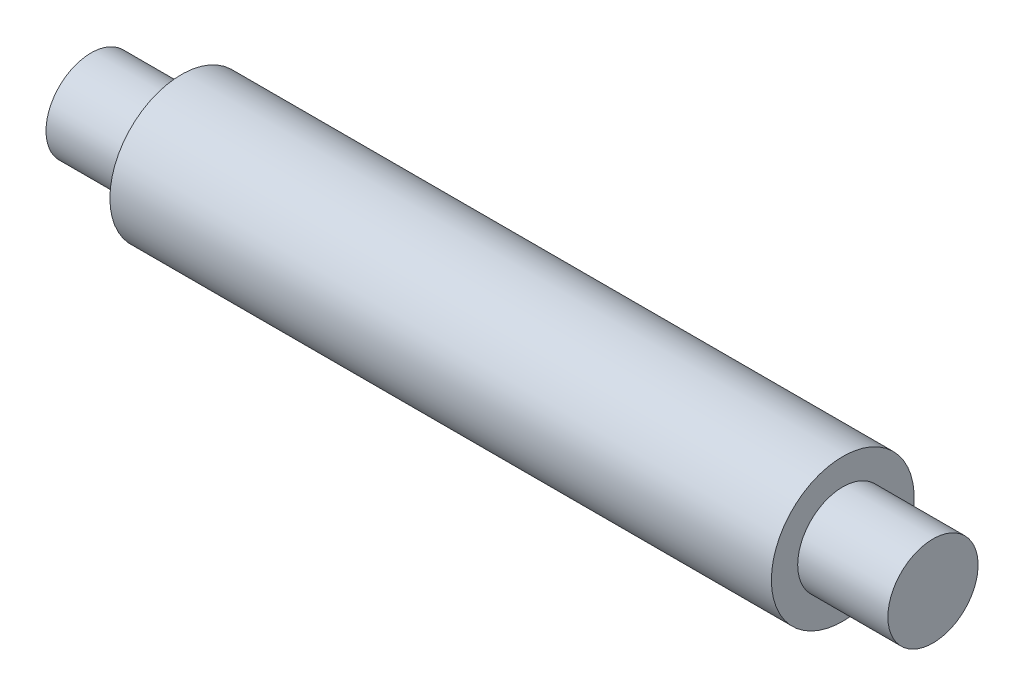
ISO-10303-21;
HEADER;
FILE_DESCRIPTION(('STEP AP214'),'2;1');
FILE_NAME('part.step','',(''),(''),'','','');
FILE_SCHEMA(('AUTOMOTIVE_DESIGN { 1 0 10303 214 1 1 1 1 }'));
ENDSEC;
DATA;
#1=APPLICATION_CONTEXT('core data for automotive mechanical design processes');
#2=APPLICATION_PROTOCOL_DEFINITION('international standard','automotive_design',2000,#1);
#3=PRODUCT_CONTEXT('',#1,'mechanical');
#4=PRODUCT('Part','Part','',(#3));
#5=PRODUCT_RELATED_PRODUCT_CATEGORY('part','',(#4));
#6=PRODUCT_DEFINITION_FORMATION('','',#4);
#7=PRODUCT_DEFINITION_CONTEXT('part definition',#1,'design');
#8=PRODUCT_DEFINITION('design','',#6,#7);
#9=PRODUCT_DEFINITION_SHAPE('','',#8);
#10=(LENGTH_UNIT() NAMED_UNIT(*) SI_UNIT(.MILLI.,.METRE.));
#11=(NAMED_UNIT(*) PLANE_ANGLE_UNIT() SI_UNIT($,.RADIAN.));
#12=(NAMED_UNIT(*) SI_UNIT($,.STERADIAN.) SOLID_ANGLE_UNIT());
#13=UNCERTAINTY_MEASURE_WITH_UNIT(LENGTH_MEASURE(1.E-05),#10,'distance_accuracy_value','');
#14=(GEOMETRIC_REPRESENTATION_CONTEXT(3) GLOBAL_UNCERTAINTY_ASSIGNED_CONTEXT((#13)) GLOBAL_UNIT_ASSIGNED_CONTEXT((#10,
#11,#12)) REPRESENTATION_CONTEXT('',''));
#15=CARTESIAN_POINT('',(0.,0.,0.));
#16=DIRECTION('',(0.,0.,1.));
#17=DIRECTION('',(1.,0.,0.));
#18=AXIS2_PLACEMENT_3D('',#15,#16,#17);
#19=CARTESIAN_POINT('',(280.,30.0000000000002,0.));
#20=DIRECTION('',(1.,0.,0.));
#21=DIRECTION('',(0.,0.,-1.));
#22=AXIS2_PLACEMENT_3D('',#19,#20,#21);
#23=PLANE('',#22);
#24=CARTESIAN_POINT('',(280.,0.,0.));
#25=DIRECTION('',(-1.,0.,0.));
#26=DIRECTION('',(0.,0.,1.));
#27=AXIS2_PLACEMENT_3D('',#24,#25,#26);
#28=CIRCLE('',#27,30.0000000000002);
#29=CARTESIAN_POINT('',(280.,0.,30.0000000000002));
#30=VERTEX_POINT('',#29);
#31=EDGE_CURVE('E10',#30,#30,#28,.T.);
#32=ORIENTED_EDGE('',*,*,#31,.F.);
#33=EDGE_LOOP('',(#32));
#34=FACE_BOUND('',#33,.T.);
#35=ADVANCED_FACE('F36',(#34),#23,.T.);
#36=CARTESIAN_POINT('',(-409.616293782747,0.,0.));
#37=DIRECTION('',(-1.,0.,0.));
#38=DIRECTION('',(0.,0.,1.));
#39=AXIS2_PLACEMENT_3D('',#36,#37,#38);
#40=CYLINDRICAL_SURFACE('',#39,30.0000000000002);
#41=ORIENTED_EDGE('',*,*,#31,.T.);
#42=EDGE_LOOP('',(#41));
#43=FACE_BOUND('',#42,.T.);
#44=CARTESIAN_POINT('',(220.,0.,0.));
#45=DIRECTION('',(-1.,0.,0.));
#46=DIRECTION('',(0.,0.,1.));
#47=AXIS2_PLACEMENT_3D('',#44,#45,#46);
#48=CIRCLE('',#47,30.0000000000002);
#49=CARTESIAN_POINT('',(220.,0.,30.0000000000002));
#50=VERTEX_POINT('',#49);
#51=EDGE_CURVE('E46',#50,#50,#48,.T.);
#52=ORIENTED_EDGE('',*,*,#51,.F.);
#53=EDGE_LOOP('',(#52));
#54=FACE_BOUND('',#53,.T.);
#55=ADVANCED_FACE('F142',(#43,#54),#40,.T.);
#56=CARTESIAN_POINT('',(220.,47.5000000000001,0.));
#57=DIRECTION('',(1.,0.,0.));
#58=DIRECTION('',(0.,0.,-1.));
#59=AXIS2_PLACEMENT_3D('',#56,#57,#58);
#60=PLANE('',#59);
#61=ORIENTED_EDGE('',*,*,#51,.T.);
#62=EDGE_LOOP('',(#61));
#63=FACE_BOUND('',#62,.T.);
#64=CARTESIAN_POINT('',(220.,0.,0.));
#65=DIRECTION('',(-1.,0.,0.));
#66=DIRECTION('',(0.,0.,1.));
#67=AXIS2_PLACEMENT_3D('',#64,#65,#66);
#68=CIRCLE('',#67,47.5000000000001);
#69=CARTESIAN_POINT('',(220.,0.,47.5000000000001));
#70=VERTEX_POINT('',#69);
#71=EDGE_CURVE('E49',#70,#70,#68,.T.);
#72=ORIENTED_EDGE('',*,*,#71,.F.);
#73=EDGE_LOOP('',(#72));
#74=FACE_BOUND('',#73,.T.);
#75=ADVANCED_FACE('F138',(#63,#74),#60,.T.);
#76=CARTESIAN_POINT('',(-409.616293782747,0.,0.));
#77=DIRECTION('',(-1.,0.,0.));
#78=DIRECTION('',(0.,0.,1.));
#79=AXIS2_PLACEMENT_3D('',#76,#77,#78);
#80=CYLINDRICAL_SURFACE('',#79,47.5);
#81=ORIENTED_EDGE('',*,*,#71,.T.);
#82=EDGE_LOOP('',(#81));
#83=FACE_BOUND('',#82,.T.);
#84=CARTESIAN_POINT('',(-220.,0.,0.));
#85=DIRECTION('',(-1.,0.,0.));
#86=DIRECTION('',(0.,0.,1.));
#87=AXIS2_PLACEMENT_3D('',#84,#85,#86);
#88=CIRCLE('',#87,47.4999999999999);
#89=CARTESIAN_POINT('',(-220.,0.,47.4999999999999));
#90=VERTEX_POINT('',#89);
#91=EDGE_CURVE('E53',#90,#90,#88,.T.);
#92=ORIENTED_EDGE('',*,*,#91,.F.);
#93=EDGE_LOOP('',(#92));
#94=FACE_BOUND('',#93,.T.);
#95=ADVANCED_FACE('F133',(#83,#94),#80,.T.);
#96=CARTESIAN_POINT('',(-220.,47.4999999999999,0.));
#97=DIRECTION('',(-1.,0.,0.));
#98=DIRECTION('',(0.,0.,1.));
#99=AXIS2_PLACEMENT_3D('',#96,#97,#98);
#100=PLANE('',#99);
#101=ORIENTED_EDGE('',*,*,#91,.T.);
#102=EDGE_LOOP('',(#101));
#103=FACE_BOUND('',#102,.T.);
#104=CARTESIAN_POINT('',(-220.,0.,0.));
#105=DIRECTION('',(-1.,0.,0.));
#106=DIRECTION('',(0.,0.,1.));
#107=AXIS2_PLACEMENT_3D('',#104,#105,#106);
#108=CIRCLE('',#107,29.9999999999999);
#109=CARTESIAN_POINT('',(-220.,0.,29.9999999999999));
#110=VERTEX_POINT('',#109);
#111=EDGE_CURVE('E56',#110,#110,#108,.T.);
#112=ORIENTED_EDGE('',*,*,#111,.F.);
#113=EDGE_LOOP('',(#112));
#114=FACE_BOUND('',#113,.T.);
#115=ADVANCED_FACE('F128',(#103,#114),#100,.T.);
#116=CARTESIAN_POINT('',(-409.616293782747,0.,0.));
#117=DIRECTION('',(-1.,0.,0.));
#118=DIRECTION('',(0.,0.,1.));
#119=AXIS2_PLACEMENT_3D('',#116,#117,#118);
#120=CYLINDRICAL_SURFACE('',#119,29.9999999999999);
#121=ORIENTED_EDGE('',*,*,#111,.T.);
#122=EDGE_LOOP('',(#121));
#123=FACE_BOUND('',#122,.T.);
#124=CARTESIAN_POINT('',(-280.,0.,0.));
#125=DIRECTION('',(-1.,0.,0.));
#126=DIRECTION('',(0.,0.,1.));
#127=AXIS2_PLACEMENT_3D('',#124,#125,#126);
#128=CIRCLE('',#127,29.9999999999999);
#129=CARTESIAN_POINT('',(-280.,0.,29.9999999999999));
#130=VERTEX_POINT('',#129);
#131=EDGE_CURVE('E65',#130,#130,#128,.T.);
#132=ORIENTED_EDGE('',*,*,#131,.F.);
#133=EDGE_LOOP('',(#132));
#134=FACE_BOUND('',#133,.T.);
#135=ADVANCED_FACE('F127',(#123,#134),#120,.T.);
#136=CARTESIAN_POINT('',(-280.,29.9999999999999,0.));
#137=DIRECTION('',(-1.,0.,0.));
#138=DIRECTION('',(0.,0.,1.));
#139=AXIS2_PLACEMENT_3D('',#136,#137,#138);
#140=PLANE('',#139);
#141=ORIENTED_EDGE('',*,*,#131,.T.);
#142=EDGE_LOOP('',(#141));
#143=FACE_BOUND('',#142,.T.);
#144=ADVANCED_FACE('F123',(#143),#140,.T.);
#145=CLOSED_SHELL('',(#35,#55,#75,#95,#115,#135,#144));
#146=CARTESIAN_POINT('',(270.,30.0000000000002,0.));
#147=DIRECTION('',(1.,0.,0.));
#148=DIRECTION('',(0.,0.,-1.));
#149=AXIS2_PLACEMENT_3D('',#146,#147,#148);
#150=PLANE('',#149);
#151=CARTESIAN_POINT('',(270.,0.,0.));
#152=DIRECTION('',(-1.,0.,0.));
#153=DIRECTION('',(0.,0.,1.));
#154=AXIS2_PLACEMENT_3D('',#151,#152,#153);
#155=CIRCLE('',#154,20.0000000000002);
#156=CARTESIAN_POINT('',(270.,0.,20.0000000000002));
#157=VERTEX_POINT('',#156);
#158=EDGE_CURVE('E79',#157,#157,#155,.T.);
#159=ORIENTED_EDGE('',*,*,#158,.T.);
#160=EDGE_LOOP('',(#159));
#161=FACE_BOUND('',#160,.T.);
#162=ADVANCED_FACE('F37',(#161),#150,.F.);
#163=CARTESIAN_POINT('',(-270.,29.9999999999999,0.));
#164=DIRECTION('',(-1.,0.,0.));
#165=DIRECTION('',(0.,0.,1.));
#166=AXIS2_PLACEMENT_3D('',#163,#164,#165);
#167=PLANE('',#166);
#168=CARTESIAN_POINT('',(-270.,0.,0.));
#169=DIRECTION('',(-1.,0.,0.));
#170=DIRECTION('',(0.,0.,1.));
#171=AXIS2_PLACEMENT_3D('',#168,#169,#170);
#172=CIRCLE('',#171,19.9999999999999);
#173=CARTESIAN_POINT('',(-270.,0.,19.9999999999999));
#174=VERTEX_POINT('',#173);
#175=EDGE_CURVE('E64',#174,#174,#172,.T.);
#176=ORIENTED_EDGE('',*,*,#175,.F.);
#177=EDGE_LOOP('',(#176));
#178=FACE_BOUND('',#177,.T.);
#179=ADVANCED_FACE('F114',(#178),#167,.F.);
#180=CARTESIAN_POINT('',(-409.616293782747,0.,0.));
#181=DIRECTION('',(-1.,0.,0.));
#182=DIRECTION('',(0.,0.,1.));
#183=AXIS2_PLACEMENT_3D('',#180,#181,#182);
#184=CYLINDRICAL_SURFACE('',#183,19.9999999999999);
#185=CARTESIAN_POINT('',(-210.,0.,0.));
#186=DIRECTION('',(-1.,0.,0.));
#187=DIRECTION('',(0.,0.,1.));
#188=AXIS2_PLACEMENT_3D('',#185,#186,#187);
#189=CIRCLE('',#188,19.9999999999999);
#190=CARTESIAN_POINT('',(-210.,0.,19.9999999999999));
#191=VERTEX_POINT('',#190);
#192=EDGE_CURVE('E68',#191,#191,#189,.T.);
#193=ORIENTED_EDGE('',*,*,#192,.F.);
#194=EDGE_LOOP('',(#193));
#195=FACE_BOUND('',#194,.T.);
#196=ORIENTED_EDGE('',*,*,#175,.T.);
#197=EDGE_LOOP('',(#196));
#198=FACE_BOUND('',#197,.T.);
#199=ADVANCED_FACE('F110',(#195,#198),#184,.F.);
#200=CARTESIAN_POINT('',(-210.,47.4999999999999,0.));
#201=DIRECTION('',(-1.,0.,0.));
#202=DIRECTION('',(0.,0.,1.));
#203=AXIS2_PLACEMENT_3D('',#200,#201,#202);
#204=PLANE('',#203);
#205=CARTESIAN_POINT('',(-210.,0.,0.));
#206=DIRECTION('',(-1.,0.,0.));
#207=DIRECTION('',(0.,0.,1.));
#208=AXIS2_PLACEMENT_3D('',#205,#206,#207);
#209=CIRCLE('',#208,37.4999999999999);
#210=CARTESIAN_POINT('',(-210.,0.,37.4999999999999));
#211=VERTEX_POINT('',#210);
#212=EDGE_CURVE('E72',#211,#211,#209,.T.);
#213=ORIENTED_EDGE('',*,*,#212,.F.);
#214=EDGE_LOOP('',(#213));
#215=FACE_BOUND('',#214,.T.);
#216=ORIENTED_EDGE('',*,*,#192,.T.);
#217=EDGE_LOOP('',(#216));
#218=FACE_BOUND('',#217,.T.);
#219=ADVANCED_FACE('F101',(#215,#218),#204,.F.);
#220=CARTESIAN_POINT('',(-409.616293782747,0.,0.));
#221=DIRECTION('',(-1.,0.,0.));
#222=DIRECTION('',(0.,0.,1.));
#223=AXIS2_PLACEMENT_3D('',#220,#221,#222);
#224=CYLINDRICAL_SURFACE('',#223,37.5);
#225=CARTESIAN_POINT('',(210.,0.,0.));
#226=DIRECTION('',(-1.,0.,0.));
#227=DIRECTION('',(0.,0.,1.));
#228=AXIS2_PLACEMENT_3D('',#225,#226,#227);
#229=CIRCLE('',#228,37.5000000000001);
#230=CARTESIAN_POINT('',(210.,0.,37.5000000000001));
#231=VERTEX_POINT('',#230);
#232=EDGE_CURVE('E74',#231,#231,#229,.T.);
#233=ORIENTED_EDGE('',*,*,#232,.F.);
#234=EDGE_LOOP('',(#233));
#235=FACE_BOUND('',#234,.T.);
#236=ORIENTED_EDGE('',*,*,#212,.T.);
#237=EDGE_LOOP('',(#236));
#238=FACE_BOUND('',#237,.T.);
#239=ADVANCED_FACE('F92',(#235,#238),#224,.F.);
#240=CARTESIAN_POINT('',(210.,47.4999999999999,0.));
#241=DIRECTION('',(1.,0.,0.));
#242=DIRECTION('',(0.,0.,-1.));
#243=AXIS2_PLACEMENT_3D('',#240,#241,#242);
#244=PLANE('',#243);
#245=CARTESIAN_POINT('',(210.000000000001,0.,0.));
#246=DIRECTION('',(-1.,0.,0.));
#247=DIRECTION('',(0.,0.,1.));
#248=AXIS2_PLACEMENT_3D('',#245,#246,#247);
#249=CIRCLE('',#248,20.0000000000002);
#250=CARTESIAN_POINT('',(210.000000000001,0.,20.0000000000002));
#251=VERTEX_POINT('',#250);
#252=EDGE_CURVE('E80',#251,#251,#249,.T.);
#253=ORIENTED_EDGE('',*,*,#252,.F.);
#254=EDGE_LOOP('',(#253));
#255=FACE_BOUND('',#254,.T.);
#256=ORIENTED_EDGE('',*,*,#232,.T.);
#257=EDGE_LOOP('',(#256));
#258=FACE_BOUND('',#257,.T.);
#259=ADVANCED_FACE('F86',(#255,#258),#244,.F.);
#260=CARTESIAN_POINT('',(-409.616293782747,0.,0.));
#261=DIRECTION('',(-1.,0.,0.));
#262=DIRECTION('',(0.,0.,1.));
#263=AXIS2_PLACEMENT_3D('',#260,#261,#262);
#264=CYLINDRICAL_SURFACE('',#263,20.0000000000002);
#265=ORIENTED_EDGE('',*,*,#158,.F.);
#266=EDGE_LOOP('',(#265));
#267=FACE_BOUND('',#266,.T.);
#268=ORIENTED_EDGE('',*,*,#252,.T.);
#269=EDGE_LOOP('',(#268));
#270=FACE_BOUND('',#269,.T.);
#271=ADVANCED_FACE('F84',(#267,#270),#264,.F.);
#272=CLOSED_SHELL('',(#162,#179,#199,#219,#239,#259,#271));
#273=ORIENTED_CLOSED_SHELL('',*,#272,.T.);
#274=BREP_WITH_VOIDS('B2',#145,(#273));
#275=ADVANCED_BREP_SHAPE_REPRESENTATION('',(#18,#274),#14);
#276=SHAPE_DEFINITION_REPRESENTATION(#9,#275);
ENDSEC;
END-ISO-10303-21;
